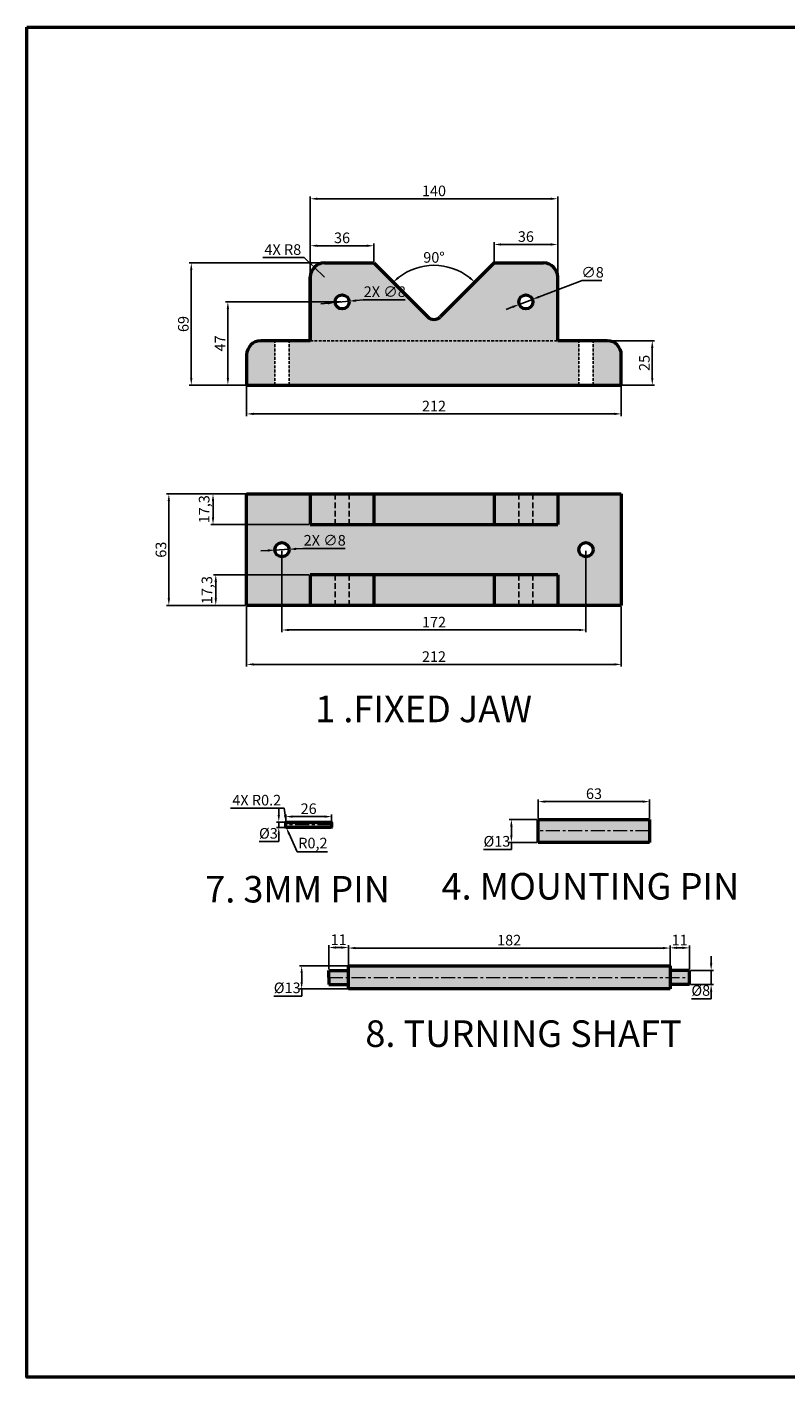
# Model space of a CAD drawing. Units: millimetres. Extents: x -14 to 1073, y -445 to 318.
# Tile 1 of 6: x -14 to 415, y -445 to 318. Entities that reach past the tile are written whole.
import ezdxf

# ---------------------------------------------------------------- set-up
doc = ezdxf.new("R2010")
doc.units = ezdxf.units.MM
doc.header["$LTSCALE"] = 0.5
doc.linetypes.add('CENTER', pattern=[50.8, 31.75, -6.35, 6.35, -6.35])
doc.linetypes.add('HIDDEN', pattern=[9.525, 6.35, -3.175])
for name, color, linetype, lineweight in [('M-CNTR', 1, 'CENTER', 18), ('M-DIMS', 2, 'Continuous', 25), ('M-HATC', 8, 'Continuous', 18), ('M-HIDN', 4, 'HIDDEN', 25), ('M-OUTL', 7, 'Continuous', 50), ('M-TEXT', 3, 'Continuous', 25)]:
    doc.layers.add(name, color=color, linetype=linetype, lineweight=lineweight)
doc.styles.get("Standard").update_dxf_attribs({"font": 'arial.ttf'})
doc.dimstyles.new('ISO-25', dxfattribs={"dimtxt": 6, "dimasz": 4, "dimexe": 1.25, "dimexo": 0.625, "dimtad": 1, "dimtoh": 1, "dimtxsty": 'Standard', "dimcen": 2.5, "dimadec": 0, "dimazin": 0, "dimtfac": 1, "dimtmove": 0, "dimatfit": 3, "dimfxl": 1, "dimarcsym": 0})

# ---------------------------------------------------------------- blocks, each defined once
blk = doc.blocks.new('*D1')
at = {"layer": 'Defpoints', "color": 0, "transparency": 16777216}
for p in [(286.52, 220.97), (146.52, 166.84), (286.52, 166.84)]:
    blk.add_point(p, dxfattribs=at)
at = {"layer": 'M-DIMS', "color": 0, "lineweight": -2, "transparency": 16777216}
for p, q in [((146.52, 167.46), (146.52, 222.22)), ((286.52, 167.46), (286.52, 222.22)), ((150.52, 220.97), (282.52, 220.97))]:
    blk.add_line(p, q, dxfattribs=at)
at = {"layer": 'M-DIMS', "color": 0, "transparency": 16777216}
for points in [[(150.52, 221.64), (150.52, 220.3), (146.52, 220.97)], [(282.52, 221.64), (282.52, 220.3), (286.52, 220.97)]]:
    blk.add_solid(points, dxfattribs=at)
at = {"layer": 'M-DIMS', "color": 0, "transparency": 16777216, "insert": (216.52, 224.66), "char_height": 6, "attachment_point": 5}
blk.add_mtext('140', dxfattribs=at)
blk = doc.blocks.new('*D2')
at = {"layer": 'Defpoints', "color": 0, "transparency": 16777216}
for p in [(146.52, 194.84), (182.52, 194.42), (182.52, 184.67)]:
    blk.add_point(p, dxfattribs=at)
at = {"layer": 'M-DIMS', "color": 0, "lineweight": -2, "transparency": 16777216}
for p, q in [((146.52, 194.22), (146.52, 193.17)), ((150.52, 194.42), (178.52, 194.42)), ((182.52, 185.29), (182.52, 195.67))]:
    blk.add_line(p, q, dxfattribs=at)
at = {"layer": 'M-DIMS', "color": 0, "transparency": 16777216}
for points in [[(150.52, 195.09), (150.52, 193.76), (146.52, 194.42)], [(178.52, 195.09), (178.52, 193.76), (182.52, 194.42)]]:
    blk.add_solid(points, dxfattribs=at)
at = {"layer": 'M-DIMS', "color": 0, "transparency": 16777216, "insert": (164.52, 198.11), "char_height": 6, "attachment_point": 5}
blk.add_mtext('36', dxfattribs=at)
blk = doc.blocks.new('*D3')
at = {"layer": 'Defpoints', "color": 0, "transparency": 16777216}
for p in [(286.52, 195.13), (250.52, 184.67), (286.52, 184.67)]:
    blk.add_point(p, dxfattribs=at)
at = {"layer": 'M-DIMS', "color": 0, "lineweight": -2, "transparency": 16777216}
for p, q in [((250.52, 185.29), (250.52, 196.38)), ((254.52, 195.13), (282.52, 195.13)), ((286.52, 185.29), (286.52, 196.38))]:
    blk.add_line(p, q, dxfattribs=at)
at = {"layer": 'M-DIMS', "color": 0, "transparency": 16777216}
for points in [[(254.52, 195.8), (254.52, 194.47), (250.52, 195.13)], [(282.52, 195.8), (282.52, 194.47), (286.52, 195.13)]]:
    blk.add_solid(points, dxfattribs=at)
at = {"layer": 'M-DIMS', "color": 0, "transparency": 16777216, "insert": (268.52, 198.82), "char_height": 6, "attachment_point": 5}
blk.add_mtext('36', dxfattribs=at)
blk = doc.blocks.new('*D4')
at = {"layer": 'Defpoints', "color": 0, "transparency": 16777216}
for p in [(110.52, 115.67), (322.52, 115.67), (322.52, 99.35)]:
    blk.add_point(p, dxfattribs=at)
at = {"layer": 'M-DIMS', "color": 0, "lineweight": -2, "transparency": 16777216}
for p, q in [((110.52, 115.04), (110.52, 98.1)), ((322.52, 115.04), (322.52, 98.1)), ((114.52, 99.35), (318.52, 99.35))]:
    blk.add_line(p, q, dxfattribs=at)
at = {"layer": 'M-DIMS', "color": 0, "transparency": 16777216}
for points in [[(114.52, 100.02), (114.52, 98.68), (110.52, 99.35)], [(318.52, 100.02), (318.52, 98.68), (322.52, 99.35)]]:
    blk.add_solid(points, dxfattribs=at)
at = {"layer": 'M-DIMS', "color": 0, "transparency": 16777216, "insert": (216.52, 102.99), "char_height": 6, "attachment_point": 5}
blk.add_mtext('212', dxfattribs=at)
blk = doc.blocks.new('*D5')
at = {"layer": 'Defpoints', "color": 0, "transparency": 16777216}
for p in [(307.53, 140.67), (307.53, 115.67), (340.04, 115.67)]:
    blk.add_point(p, dxfattribs=at)
at = {"layer": 'M-DIMS', "color": 0, "lineweight": -2, "transparency": 16777216}
for p, q in [((308.16, 140.67), (341.29, 140.67)), ((340.04, 136.67), (340.04, 119.67)), ((308.16, 115.67), (341.29, 115.67))]:
    blk.add_line(p, q, dxfattribs=at)
at = {"layer": 'M-DIMS', "color": 0, "transparency": 16777216}
for points in [[(339.37, 136.67), (340.7, 136.67), (340.04, 140.67)], [(339.37, 119.67), (340.7, 119.67), (340.04, 115.67)]]:
    blk.add_solid(points, dxfattribs=at)
at = {"layer": 'M-DIMS', "color": 0, "transparency": 16777216, "insert": (336.35, 128.17), "char_height": 6, "attachment_point": 5, "rotation": 90}
blk.add_mtext('25', dxfattribs=at)
blk = doc.blocks.new('*D6')
at = {"layer": 'Defpoints', "color": 0, "transparency": 16777216}
for p in [(164.52, 162.67), (99.9, 115.67), (164.52, 115.67)]:
    blk.add_point(p, dxfattribs=at)
at = {"layer": 'M-DIMS', "color": 0, "lineweight": -2, "transparency": 16777216}
for p, q in [((163.9, 162.67), (98.65, 162.67)), ((99.9, 158.67), (99.9, 119.67)), ((163.9, 115.67), (98.65, 115.67))]:
    blk.add_line(p, q, dxfattribs=at)
at = {"layer": 'M-DIMS', "color": 0, "transparency": 16777216}
for points in [[(99.24, 158.67), (100.57, 158.67), (99.9, 162.67)], [(99.24, 119.67), (100.57, 119.67), (99.9, 115.67)]]:
    blk.add_solid(points, dxfattribs=at)
at = {"layer": 'M-DIMS', "color": 0, "transparency": 16777216, "insert": (96.28, 139.17), "char_height": 6, "attachment_point": 5, "rotation": 90}
blk.add_mtext('47', dxfattribs=at)
blk = doc.blocks.new('*D7')
at = {"layer": 'Defpoints', "color": 0, "transparency": 16777216}
for p in [(168.52, 184.67), (79.19, 115.67), (168.52, 115.67)]:
    blk.add_point(p, dxfattribs=at)
at = {"layer": 'M-DIMS', "color": 0, "lineweight": -2, "transparency": 16777216}
for p, q in [((167.9, 184.67), (77.94, 184.67)), ((79.19, 180.67), (79.19, 119.67)), ((167.9, 115.67), (77.94, 115.67))]:
    blk.add_line(p, q, dxfattribs=at)
at = {"layer": 'M-DIMS', "color": 0, "transparency": 16777216}
for points in [[(78.52, 180.67), (79.85, 180.67), (79.19, 184.67)], [(78.52, 119.67), (79.85, 119.67), (79.19, 115.67)]]:
    blk.add_solid(points, dxfattribs=at)
at = {"layer": 'M-DIMS', "color": 0, "transparency": 16777216, "insert": (75.5, 150.17), "char_height": 6, "attachment_point": 5, "rotation": 90}
blk.add_mtext('69', dxfattribs=at)
blk = doc.blocks.new('*D8')
at = {"layer": 'Defpoints', "color": 0, "transparency": 16777216}
for p in [(182.52, 184.67), (250.52, 184.67), (224.98, 182.24), (212.99, 154.2), (220.06, 154.2)]:
    blk.add_point(p, dxfattribs=at)
at = {"layer": 'M-DIMS', "color": 0, "lineweight": -2, "transparency": 16777216}
blk.add_arc((216.52, 150.67), 32.69, 52.01622, 127.98378, dxfattribs=at)
at = {"layer": 'M-DIMS', "color": 0, "transparency": 16777216}
for points in [[(196.85, 175.93), (195.96, 176.93), (193.41, 173.78)], [(237.08, 176.93), (236.2, 175.93), (239.63, 173.78)]]:
    blk.add_solid(points, dxfattribs=at)
at = {"layer": 'M-DIMS', "color": 0, "transparency": 16777216, "insert": (216.52, 187.04), "char_height": 6, "attachment_point": 5}
blk.add_mtext('90°', dxfattribs=at)
blk = doc.blocks.new('*D9')
at = {"layer": 'Defpoints', "color": 0, "transparency": 16777216}
for p in [(264.78, 161.25), (272.26, 164.09)]:
    blk.add_point(p, dxfattribs=at)
at = {"layer": 'M-DIMS', "color": 0, "lineweight": -2, "transparency": 16777216}
for p, q in [((300.4, 174.76), (276, 165.5)), ((311.5, 174.76), (300.4, 174.76)), ((264.78, 161.25), (272.26, 164.09)), ((261.04, 159.83), (257.3, 158.41))]:
    blk.add_line(p, q, dxfattribs=at)
at = {"layer": 'M-DIMS', "color": 0, "transparency": 16777216}
for points in [[(260.81, 160.45), (261.28, 159.21), (264.78, 161.25)], [(275.77, 166.13), (276.24, 164.88), (272.26, 164.09)]]:
    blk.add_solid(points, dxfattribs=at)
at = {"layer": 'M-DIMS', "color": 0, "transparency": 16777216, "insert": (306.26, 178.61), "char_height": 6, "attachment_point": 5}
blk.add_mtext('∅8', dxfattribs=at)
blk = doc.blocks.new('*D10')
at = {"layer": 'Defpoints', "color": 0, "ltscale": 0.5, "transparency": 16777216}
for p in [(110.52, -8.93), (322.52, -8.93), (322.52, -42.29)]:
    blk.add_point(p, dxfattribs=at)
at = {"layer": 'M-DIMS', "color": 0, "lineweight": -2, "ltscale": 0.5, "transparency": 16777216}
for p, q in [((110.52, -9.55), (110.52, -43.54)), ((322.52, -9.55), (322.52, -43.54)), ((114.52, -42.29), (318.52, -42.29))]:
    blk.add_line(p, q, dxfattribs=at)
at = {"layer": 'M-DIMS', "color": 0, "ltscale": 0.5, "transparency": 16777216}
for points in [[(114.52, -41.63), (114.52, -42.96), (110.52, -42.29)], [(318.52, -41.63), (318.52, -42.96), (322.52, -42.29)]]:
    blk.add_solid(points, dxfattribs=at)
at = {"layer": 'M-DIMS', "color": 0, "ltscale": 0.5, "transparency": 16777216, "insert": (216.52, -38.66), "char_height": 6, "attachment_point": 5}
blk.add_mtext('212', dxfattribs=at)
blk = doc.blocks.new('*D11')
at = {"layer": 'Defpoints', "color": 0, "ltscale": 0.5, "transparency": 16777216}
for p in [(130.52, 22.57), (302.52, 22.57), (302.52, -22.83)]:
    blk.add_point(p, dxfattribs=at)
at = {"layer": 'M-DIMS', "color": 0, "lineweight": -2, "ltscale": 0.5, "transparency": 16777216}
for p, q in [((130.52, 21.95), (130.52, -24.08)), ((302.52, 21.95), (302.52, -24.08)), ((134.52, -22.83), (298.52, -22.83))]:
    blk.add_line(p, q, dxfattribs=at)
at = {"layer": 'M-DIMS', "color": 0, "ltscale": 0.5, "transparency": 16777216}
for points in [[(134.52, -22.16), (134.52, -23.49), (130.52, -22.83)], [(298.52, -22.16), (298.52, -23.49), (302.52, -22.83)]]:
    blk.add_solid(points, dxfattribs=at)
at = {"layer": 'M-DIMS', "color": 0, "ltscale": 0.5, "transparency": 16777216, "insert": (216.52, -19.19), "char_height": 6, "attachment_point": 5}
blk.add_mtext('172', dxfattribs=at)
blk = doc.blocks.new('*D12')
at = {"layer": 'Defpoints', "color": 0, "ltscale": 0.5, "transparency": 16777216}
for p in [(110.52, 54.07), (66.5, -8.93), (110.52, -8.93)]:
    blk.add_point(p, dxfattribs=at)
at = {"layer": 'M-DIMS', "color": 0, "lineweight": -2, "ltscale": 0.5, "transparency": 16777216}
for p, q in [((109.9, 54.07), (65.25, 54.07)), ((66.5, 50.07), (66.5, -4.93)), ((109.9, -8.93), (65.25, -8.93))]:
    blk.add_line(p, q, dxfattribs=at)
at = {"layer": 'M-DIMS', "color": 0, "ltscale": 0.5, "transparency": 16777216}
for points in [[(65.84, 50.07), (67.17, 50.07), (66.5, 54.07)], [(65.84, -4.93), (67.17, -4.93), (66.5, -8.93)]]:
    blk.add_solid(points, dxfattribs=at)
at = {"layer": 'M-DIMS', "color": 0, "ltscale": 0.5, "transparency": 16777216, "insert": (62.81, 22.57), "char_height": 6, "attachment_point": 5, "rotation": 90}
blk.add_mtext('63', dxfattribs=at)
blk = doc.blocks.new('*D13')
at = {"layer": 'Defpoints', "color": 0, "ltscale": 0.5, "transparency": 16777216}
for p in [(146.52, 54.07), (91.5, 36.77), (146.52, 36.77)]:
    blk.add_point(p, dxfattribs=at)
at = {"layer": 'M-DIMS', "color": 0, "lineweight": -2, "ltscale": 0.5, "transparency": 16777216}
for p, q in [((145.9, 54.07), (90.25, 54.07)), ((91.5, 50.07), (91.5, 40.77)), ((145.9, 36.77), (90.25, 36.77))]:
    blk.add_line(p, q, dxfattribs=at)
at = {"layer": 'M-DIMS', "color": 0, "ltscale": 0.5, "transparency": 16777216}
for points in [[(90.83, 50.07), (92.16, 50.07), (91.5, 54.07)], [(90.83, 40.77), (92.16, 40.77), (91.5, 36.77)]]:
    blk.add_solid(points, dxfattribs=at)
at = {"layer": 'M-DIMS', "color": 0, "ltscale": 0.5, "transparency": 16777216, "insert": (87.27, 45.42), "char_height": 6, "attachment_point": 5, "rotation": 90}
blk.add_mtext('17,3', dxfattribs=at)
blk = doc.blocks.new('*D14')
at = {"layer": 'Defpoints', "color": 0, "ltscale": 0.5, "transparency": 16777216}
for p in [(146.52, 8.37), (93.06, -8.93), (110.52, -8.93)]:
    blk.add_point(p, dxfattribs=at)
at = {"layer": 'M-DIMS', "color": 0, "lineweight": -2, "ltscale": 0.5, "transparency": 16777216}
for p, q in [((145.9, 8.37), (91.81, 8.37)), ((93.06, 4.37), (93.06, -4.93)), ((109.9, -8.93), (91.81, -8.93))]:
    blk.add_line(p, q, dxfattribs=at)
at = {"layer": 'M-DIMS', "color": 0, "ltscale": 0.5, "transparency": 16777216}
for points in [[(92.39, 4.37), (93.73, 4.37), (93.06, 8.37)], [(92.39, -4.93), (93.73, -4.93), (93.06, -8.93)]]:
    blk.add_solid(points, dxfattribs=at)
at = {"layer": 'M-DIMS', "color": 0, "ltscale": 0.5, "transparency": 16777216, "insert": (88.83, -0.28), "char_height": 6, "attachment_point": 5, "rotation": 90}
blk.add_mtext('17,3', dxfattribs=at)
blk = doc.blocks.new('*D28')
at = {"layer": 'Defpoints', "color": 0, "ltscale": 0.5, "transparency": 16777216}
for p in [(158.61, -128.34), (132.61, -132.94), (158.61, -132.94)]:
    blk.add_point(p, dxfattribs=at)
at = {"layer": 'M-DIMS', "color": 0, "lineweight": -2, "ltscale": 0.5, "transparency": 16777216}
for p, q in [((132.61, -132.31), (132.61, -127.09)), ((136.61, -128.34), (154.61, -128.34)), ((158.61, -132.31), (158.61, -127.09))]:
    blk.add_line(p, q, dxfattribs=at)
at = {"layer": 'M-DIMS', "color": 0, "ltscale": 0.5, "transparency": 16777216}
for points in [[(136.61, -127.68), (136.61, -129.01), (132.61, -128.34)], [(154.61, -127.68), (154.61, -129.01), (158.61, -128.34)]]:
    blk.add_solid(points, dxfattribs=at)
at = {"layer": 'M-DIMS', "color": 0, "ltscale": 0.5, "transparency": 16777216, "insert": (145.61, -124.65), "char_height": 6, "attachment_point": 5}
blk.add_mtext('26', dxfattribs=at)
blk = doc.blocks.new('*D29')
at = {"layer": 'Defpoints', "color": 0, "ltscale": 0.5, "transparency": 16777216}
for p in [(128.7, -134.44), (133.54, -131.44), (133.54, -134.44)]:
    blk.add_point(p, dxfattribs=at)
at = {"layer": 'M-DIMS', "color": 0, "lineweight": -2, "ltscale": 0.5, "transparency": 16777216}
for p, q in [((128.7, -127.44), (128.7, -123.44)), ((132.91, -131.44), (127.45, -131.44)), ((132.91, -134.44), (127.45, -134.44)), ((128.7, -131.44), (128.7, -134.44)), ((128.7, -142.44), (117.61, -142.44)), ((128.7, -138.44), (128.7, -142.44))]:
    blk.add_line(p, q, dxfattribs=at)
at = {"layer": 'M-DIMS', "color": 0, "ltscale": 0.5, "transparency": 16777216}
for points in [[(128.03, -127.44), (129.36, -127.44), (128.7, -131.44)], [(128.03, -138.44), (129.36, -138.44), (128.7, -134.44)]]:
    blk.add_solid(points, dxfattribs=at)
at = {"layer": 'M-DIMS', "color": 0, "ltscale": 0.5, "transparency": 16777216, "insert": (122.84, -138.58), "char_height": 6, "attachment_point": 5}
blk.add_mtext('%%C3', dxfattribs=at)
blk = doc.blocks.new('*D30')
at = {"layer": 'Defpoints', "color": 0, "ltscale": 0.5, "transparency": 16777216}
for p in [(132.81, -134.24), (132.89, -134.42)]:
    blk.add_point(p, dxfattribs=at)
at = {"layer": 'M-DIMS', "color": 0, "lineweight": -2, "ltscale": 0.5, "transparency": 16777216}
for p, q in [((132.81, -134.24), (132.89, -134.42)), ((139.09, -148.31), (134.52, -138.07)), ((156.32, -148.31), (139.09, -148.31))]:
    blk.add_line(p, q, dxfattribs=at)
blk.add_arc((132.81, -134.24), 0.2, 270, 294.08317, dxfattribs=at)
at = {"layer": 'M-DIMS', "color": 0, "ltscale": 0.5, "transparency": 16777216}
blk.add_solid([(135.13, -137.8), (133.91, -138.35), (132.89, -134.42)], dxfattribs=at)
at = {"layer": 'M-DIMS', "color": 0, "ltscale": 0.5, "transparency": 16777216, "insert": (148.02, -144.08), "char_height": 6, "attachment_point": 5}
blk.add_mtext('R0,2', dxfattribs=at)
blk = doc.blocks.new('*D31')
at = {"layer": 'Defpoints', "color": 0, "ltscale": 0.5, "transparency": 16777216}
for p in [(338.56, -119.86), (275.56, -129.94), (338.56, -129.94)]:
    blk.add_point(p, dxfattribs=at)
at = {"layer": 'M-DIMS', "color": 0, "lineweight": -2, "ltscale": 0.5, "transparency": 16777216}
for p, q in [((275.56, -129.32), (275.56, -118.61)), ((279.56, -119.86), (334.56, -119.86)), ((338.56, -129.32), (338.56, -118.61))]:
    blk.add_line(p, q, dxfattribs=at)
at = {"layer": 'M-DIMS', "color": 0, "ltscale": 0.5, "transparency": 16777216}
for points in [[(279.56, -119.2), (279.56, -120.53), (275.56, -119.86)], [(334.56, -119.2), (334.56, -120.53), (338.56, -119.86)]]:
    blk.add_solid(points, dxfattribs=at)
at = {"layer": 'M-DIMS', "color": 0, "ltscale": 0.5, "transparency": 16777216, "insert": (307.06, -116.17), "char_height": 6, "attachment_point": 5}
blk.add_mtext('63', dxfattribs=at)
blk = doc.blocks.new('*D32')
at = {"layer": 'Defpoints', "color": 0, "ltscale": 0.5, "transparency": 16777216}
for p in [(275.56, -129.94), (260.32, -142.94), (275.56, -142.94)]:
    blk.add_point(p, dxfattribs=at)
at = {"layer": 'M-DIMS', "color": 0, "lineweight": -2, "ltscale": 0.5, "transparency": 16777216}
for p, q in [((274.94, -129.94), (259.07, -129.94)), ((260.32, -133.94), (260.32, -138.94)), ((274.94, -142.94), (259.07, -142.94)), ((260.32, -142.94), (260.32, -146.94)), ((260.32, -146.94), (244.57, -146.94))]:
    blk.add_line(p, q, dxfattribs=at)
at = {"layer": 'M-DIMS', "color": 0, "ltscale": 0.5, "transparency": 16777216}
for points in [[(259.65, -133.94), (260.99, -133.94), (260.32, -129.94)], [(259.65, -138.94), (260.99, -138.94), (260.32, -142.94)]]:
    blk.add_solid(points, dxfattribs=at)
at = {"layer": 'M-DIMS', "color": 0, "ltscale": 0.5, "transparency": 16777216, "insert": (252.13, -143.08), "char_height": 6, "attachment_point": 5}
blk.add_mtext('%%C13', dxfattribs=at)
blk = doc.blocks.new('*D33')
at = {"layer": 'Defpoints', "color": 0, "ltscale": 0.5, "transparency": 16777216}
for p in [(168.07, -202.36), (157.07, -215.28), (168.07, -215.28)]:
    blk.add_point(p, dxfattribs=at)
at = {"layer": 'M-DIMS', "color": 0, "lineweight": -2, "ltscale": 0.5, "transparency": 16777216}
for p, q in [((157.07, -214.66), (157.07, -201.11)), ((161.07, -202.36), (164.07, -202.36)), ((168.07, -214.66), (168.07, -201.11))]:
    blk.add_line(p, q, dxfattribs=at)
at = {"layer": 'M-DIMS', "color": 0, "ltscale": 0.5, "transparency": 16777216}
for points in [[(161.07, -201.7), (161.07, -203.03), (157.07, -202.36)], [(164.07, -201.7), (164.07, -203.03), (168.07, -202.36)]]:
    blk.add_solid(points, dxfattribs=at)
at = {"layer": 'M-DIMS', "color": 0, "ltscale": 0.5, "transparency": 16777216, "insert": (162.57, -198.73), "char_height": 6, "attachment_point": 5}
blk.add_mtext('11', dxfattribs=at)
blk = doc.blocks.new('*D34')
at = {"layer": 'Defpoints', "color": 0, "ltscale": 0.5, "transparency": 16777216}
for p in [(350.07, -202.66), (168.07, -207.89), (350.07, -212.78)]:
    blk.add_point(p, dxfattribs=at)
at = {"layer": 'M-DIMS', "color": 0, "lineweight": -2, "ltscale": 0.5, "transparency": 16777216}
for p, q in [((168.07, -207.26), (168.07, -201.41)), ((172.07, -202.66), (346.07, -202.66)), ((350.07, -212.16), (350.07, -201.41))]:
    blk.add_line(p, q, dxfattribs=at)
at = {"layer": 'M-DIMS', "color": 0, "ltscale": 0.5, "transparency": 16777216}
for points in [[(172.07, -201.99), (172.07, -203.33), (168.07, -202.66)], [(346.07, -201.99), (346.07, -203.33), (350.07, -202.66)]]:
    blk.add_solid(points, dxfattribs=at)
at = {"layer": 'M-DIMS', "color": 0, "ltscale": 0.5, "transparency": 16777216, "insert": (259.07, -198.97), "char_height": 6, "attachment_point": 5}
blk.add_mtext('182', dxfattribs=at)
blk = doc.blocks.new('*D35')
at = {"layer": 'Defpoints', "color": 0, "ltscale": 0.5, "transparency": 16777216}
for p in [(361.07, -202.54), (350.07, -215.28), (361.07, -215.28)]:
    blk.add_point(p, dxfattribs=at)
at = {"layer": 'M-DIMS', "color": 0, "lineweight": -2, "ltscale": 0.5, "transparency": 16777216}
for p, q in [((350.07, -214.66), (350.07, -201.29)), ((354.07, -202.54), (357.07, -202.54)), ((361.07, -214.66), (361.07, -201.29))]:
    blk.add_line(p, q, dxfattribs=at)
at = {"layer": 'M-DIMS', "color": 0, "ltscale": 0.5, "transparency": 16777216}
for points in [[(354.07, -201.88), (354.07, -203.21), (350.07, -202.54)], [(357.07, -201.88), (357.07, -203.21), (361.07, -202.54)]]:
    blk.add_solid(points, dxfattribs=at)
at = {"layer": 'M-DIMS', "color": 0, "ltscale": 0.5, "transparency": 16777216, "insert": (355.57, -198.9), "char_height": 6, "attachment_point": 5}
blk.add_mtext('11', dxfattribs=at)
blk = doc.blocks.new('*D36')
at = {"layer": 'Defpoints', "color": 0, "ltscale": 0.5, "transparency": 16777216}
for p in [(361.07, -215.28), (361.07, -223.28), (373.35, -223.28)]:
    blk.add_point(p, dxfattribs=at)
at = {"layer": 'M-DIMS', "color": 0, "lineweight": -2, "ltscale": 0.5, "transparency": 16777216}
for p, q in [((373.35, -211.28), (373.35, -207.28)), ((361.7, -215.28), (374.6, -215.28)), ((373.35, -215.28), (373.35, -223.28)), ((361.7, -223.28), (374.6, -223.28)), ((373.35, -227.28), (373.35, -231.28)), ((373.35, -231.28), (362.25, -231.28))]:
    blk.add_line(p, q, dxfattribs=at)
at = {"layer": 'M-DIMS', "color": 0, "ltscale": 0.5, "transparency": 16777216}
for points in [[(372.68, -211.28), (374.01, -211.28), (373.35, -215.28)], [(372.68, -227.28), (374.01, -227.28), (373.35, -223.28)]]:
    blk.add_solid(points, dxfattribs=at)
at = {"layer": 'M-DIMS', "color": 0, "ltscale": 0.5, "transparency": 16777216, "insert": (367.48, -227.43), "char_height": 6, "attachment_point": 5}
blk.add_mtext('%%C8', dxfattribs=at)
blk = doc.blocks.new('*D37')
at = {"layer": 'Defpoints', "color": 0, "ltscale": 0.5, "transparency": 16777216}
for p in [(202.48, -212.78), (141.66, -225.78), (202.48, -225.78)]:
    blk.add_point(p, dxfattribs=at)
at = {"layer": 'M-DIMS', "color": 0, "lineweight": -2, "ltscale": 0.5, "transparency": 16777216}
for p, q in [((201.85, -212.78), (140.41, -212.78)), ((141.66, -216.78), (141.66, -221.78)), ((201.85, -225.78), (140.41, -225.78)), ((141.66, -225.78), (141.66, -229.78)), ((141.66, -229.78), (125.91, -229.78))]:
    blk.add_line(p, q, dxfattribs=at)
at = {"layer": 'M-DIMS', "color": 0, "ltscale": 0.5, "transparency": 16777216}
for points in [[(140.99, -216.78), (142.33, -216.78), (141.66, -212.78)], [(140.99, -221.78), (142.33, -221.78), (141.66, -225.78)]]:
    blk.add_solid(points, dxfattribs=at)
at = {"layer": 'M-DIMS', "color": 0, "ltscale": 0.5, "transparency": 16777216, "insert": (133.47, -225.93), "char_height": 6, "attachment_point": 5}
blk.add_mtext('%%C13', dxfattribs=at)
blk = doc.blocks.new('*D81')
at = {"layer": 'Defpoints', "color": 0, "ltscale": 0.5, "transparency": 16777216}
for p in [(148.78, 182.24), (154.52, 176.67)]:
    blk.add_point(p, dxfattribs=at)
at = {"layer": 'M-DIMS', "color": 0, "lineweight": -2, "ltscale": 0.5, "transparency": 16777216}
for p, q in [((119.59, 187.81), (143.04, 187.81)), ((143.04, 187.81), (145.91, 185.02)), ((154.52, 176.67), (148.78, 182.24))]:
    blk.add_line(p, q, dxfattribs=at)
at = {"layer": 'M-DIMS', "color": 0, "ltscale": 0.5, "transparency": 16777216}
blk.add_solid([(146.37, 185.5), (145.44, 184.54), (148.78, 182.24)], dxfattribs=at)
at = {"layer": 'M-DIMS', "color": 0, "ltscale": 0.5, "transparency": 16777216, "insert": (131, 191.49), "char_height": 6, "attachment_point": 5}
blk.add_mtext('4X R8', dxfattribs=at)
blk = doc.blocks.new('*D82')
at = {"layer": 'Defpoints', "color": 0, "ltscale": 0.5, "transparency": 16777216}
for p in [(160.54, 162.29), (168.5, 163.05)]:
    blk.add_point(p, dxfattribs=at)
at = {"layer": 'M-DIMS', "color": 0, "lineweight": -2, "ltscale": 0.5, "transparency": 16777216}
for p, q in [((156.56, 161.9), (152.58, 161.52)), ((160.54, 162.29), (168.5, 163.05)), ((176.47, 163.81), (172.49, 163.43)), ((200.24, 163.81), (176.47, 163.81))]:
    blk.add_line(p, q, dxfattribs=at)
at = {"layer": 'M-DIMS', "color": 0, "ltscale": 0.5, "transparency": 16777216}
for points in [[(156.49, 162.57), (156.62, 161.24), (160.54, 162.29)], [(172.42, 164.09), (172.55, 162.77), (168.5, 163.05)]]:
    blk.add_solid(points, dxfattribs=at)
at = {"layer": 'M-DIMS', "color": 0, "ltscale": 0.5, "transparency": 16777216, "insert": (188.67, 167.67), "char_height": 6, "attachment_point": 5}
blk.add_mtext('2X ∅8', dxfattribs=at)
blk = doc.blocks.new('*D83')
at = {"layer": 'Defpoints', "color": 0, "ltscale": 0.5, "transparency": 16777216}
for p in [(126.53, 22.35), (134.52, 22.8)]:
    blk.add_point(p, dxfattribs=at)
at = {"layer": 'M-DIMS', "color": 0, "lineweight": -2, "ltscale": 0.5, "transparency": 16777216}
for p, q in [((142.5, 23.26), (138.51, 23.03)), ((166.28, 23.26), (142.5, 23.26)), ((122.53, 22.12), (118.54, 21.89)), ((126.53, 22.35), (134.52, 22.8))]:
    blk.add_line(p, q, dxfattribs=at)
at = {"layer": 'M-DIMS', "color": 0, "ltscale": 0.5, "transparency": 16777216}
for points in [[(138.47, 23.69), (138.55, 22.36), (134.52, 22.8)], [(122.5, 22.78), (122.57, 21.45), (126.53, 22.35)]]:
    blk.add_solid(points, dxfattribs=at)
at = {"layer": 'M-DIMS', "color": 0, "ltscale": 0.5, "transparency": 16777216, "insert": (154.7, 27.11), "char_height": 6, "attachment_point": 5}
blk.add_mtext('2X ∅8', dxfattribs=at)
blk = doc.blocks.new('*D96')
at = {"layer": 'Defpoints', "color": 0, "ltscale": 0.5, "transparency": 16777216}
for p in [(132.78, -131.44), (132.81, -131.64)]:
    blk.add_point(p, dxfattribs=at)
at = {"layer": 'M-DIMS', "color": 0, "lineweight": -2, "ltscale": 0.5, "transparency": 16777216}
for p, q in [((101.36, -123.51), (131.72, -123.51)), ((131.72, -123.51), (132.25, -127.48)), ((132.81, -131.64), (132.78, -131.44))]:
    blk.add_line(p, q, dxfattribs=at)
at = {"layer": 'M-DIMS', "color": 0, "ltscale": 0.5, "transparency": 16777216}
blk.add_solid([(132.91, -127.39), (131.59, -127.56), (132.78, -131.44)], dxfattribs=at)
at = {"layer": 'M-DIMS', "color": 0, "ltscale": 0.5, "transparency": 16777216, "insert": (116.23, -119.82), "char_height": 6, "attachment_point": 5}
blk.add_mtext('4X R0.2', dxfattribs=at)

msp = doc.modelspace()

# ---------------------------------------------------------------- hatches: boundary and pattern name
at = {"layer": 'M-HATC', "ltscale": 0.5}
h = msp.add_hatch(color=256, dxfattribs=at)
h.set_gradient(color1=(41, 49, 137), color2=(41, 49, 137), tint=1)
h.paths.add_polyline_path([(182.5216, 184.6668), (154.5216, 184.6668, 0.41421356), (146.5216, 176.6668), (146.5216, 140.6668), (286.5216, 140.6668), (286.5216, 176.6668, 0.41421356), (278.5216, 184.6668), (250.5216, 184.6668), (220.0571, 154.2024, -0.41421356), (212.9861, 154.2024)])
h.paths.add_polyline_path([(160.5216, 162.6668, -1), (168.5216, 162.6668, -1)], flags=16)
h.paths.add_polyline_path([(272.5216, 162.6668, -1), (264.5216, 162.6668, -1)], flags=16)
h.paths.add_polyline_path([(298.5216, 140.6668), (286.5216, 140.6668), (146.5216, 140.6668), (134.5216, 140.6668), (134.5216, 115.6668), (298.5216, 115.6668)])
h.paths.add_polyline_path([(126.5216, 140.6668), (118.5216, 140.6668, 0.41421356), (110.5216, 132.6668), (110.5216, 115.6668), (126.5216, 115.6668)])
h.paths.add_polyline_path([(322.5216, 132.6668, 0.41421356), (314.5216, 140.6668), (306.5216, 140.6668), (306.5216, 115.6668), (322.5216, 115.6668)])
h = msp.add_hatch(color=256, dxfattribs=at)
h.set_gradient(color1=(69, 84, 165), color2=(69, 84, 165), tint=1)
h.paths.add_polyline_path([(322.5216, 54.0737), (286.5216, 54.0737), (286.5216, 36.7737), (146.5216, 36.7737), (146.5216, 54.0737), (110.5216, 54.0737), (110.5216, -8.9263), (146.5216, -8.9263), (146.5216, 8.3737), (286.5216, 8.3737), (286.5216, -8.9263), (322.5216, -8.9263)])
h.paths.add_polyline_path([(306.5216, 22.5737, -1), (298.5216, 22.5737, -1)], flags=16)
h.paths.add_polyline_path([(126.5216, 22.5737, -1), (134.5216, 22.5737, -1)], flags=16)
h.paths.add_polyline_path([(250.5216, 54.0737), (182.5216, 54.0737), (182.5216, 36.7737), (250.5216, 36.7737)], flags=17)
h.paths.add_polyline_path([(182.5216, 54.0737), (168.5216, 54.0737), (168.5216, 36.7737), (182.5216, 36.7737)], flags=17)
h.paths.add_polyline_path([(168.5216, 54.0737), (160.5216, 54.0737), (160.5216, 36.7737), (168.5216, 36.7737)], flags=17)
h.paths.add_polyline_path([(160.5216, 54.0737), (146.5216, 54.0737), (146.5216, 36.7737), (160.5216, 36.7737)], flags=17)
h.paths.add_polyline_path([(264.5216, 54.0737), (250.5216, 54.0737), (250.5216, 36.7737), (264.5216, 36.7737)], flags=17)
h.paths.add_polyline_path([(272.5216, 54.0737), (264.5216, 54.0737), (264.5216, 36.7737), (272.5216, 36.7737)], flags=17)
h.paths.add_polyline_path([(286.5216, 54.0737), (272.5216, 54.0737), (272.5216, 36.7737), (286.5216, 36.7737)], flags=17)
h.paths.add_polyline_path([(160.5216, 8.3737), (146.5216, 8.3737), (146.5216, -8.9263), (160.5216, -8.9263)], flags=17)
h.paths.add_polyline_path([(168.5216, 8.3737), (160.5216, 8.3737), (160.5216, -8.9263), (168.5216, -8.9263)], flags=17)
h.paths.add_polyline_path([(182.5216, 8.3737), (168.5216, 8.3737), (168.5216, -8.9263), (182.5216, -8.9263)], flags=17)
h.paths.add_polyline_path([(250.5216, 8.3737), (182.5216, 8.3737), (182.5216, -8.9263), (250.5216, -8.9263)], flags=17)
h.paths.add_polyline_path([(264.5216, 8.3737), (250.5216, 8.3737), (250.5216, -8.9263), (264.5216, -8.9263)], flags=17)
h.paths.add_polyline_path([(272.5216, 8.3737), (264.5216, 8.3737), (264.5216, -8.9263), (272.5216, -8.9263)], flags=17)
h.paths.add_polyline_path([(286.5216, 8.3737), (272.5216, 8.3737), (272.5216, -8.9263), (286.5216, -8.9263)], flags=17)
h = msp.add_hatch(color=256, dxfattribs=at)
h.set_gradient(color1=(221, 179, 212), color2=(221, 179, 212), tint=1)
h.paths.add_polyline_path([(158.6052, -132.939), (158.6052, -131.639, 0.41421356), (158.4052, -131.439), (132.8052, -131.439, 0.41421356), (132.6052, -131.639), (132.6052, -132.939)])
h.paths.add_polyline_path([(132.6052, -132.939), (132.6052, -134.239, 0.41421356), (132.8052, -134.439), (158.4052, -134.439, 0.41421356), (158.6052, -134.239), (158.6052, -132.939)])
h = msp.add_hatch(color=256, dxfattribs=at)
h.set_gradient(color1=(128, 128, 128), color2=(128, 128, 128), tint=1)
h.paths.add_polyline_path([(338.5603, -136.4411), (275.5603, -136.4411), (275.5603, -142.9411), (338.5603, -142.9411)])
h.paths.add_polyline_path([(338.5603, -129.9411), (275.5603, -129.9411), (275.5603, -136.4411), (338.5603, -136.4411)])
h = msp.add_hatch(color=256, dxfattribs=at)
h.set_gradient(color1=(128, 128, 128), color2=(192, 192, 192), tint=1, name='INVCYLINDER')
h.paths.add_polyline_path([(350.0728, -212.7819), (168.0728, -212.7819), (168.0728, -219.2819), (350.0728, -219.2819)])
h.paths.add_polyline_path([(350.0728, -219.2819), (168.0728, -219.2819), (168.0728, -225.7819), (350.0728, -225.7819)])
h.paths.add_polyline_path([(168.0728, -215.2819), (157.0728, -215.2819), (157.0728, -219.2819), (168.0728, -219.2819)])
h.paths.add_polyline_path([(168.0728, -219.2819), (157.0728, -219.2819), (157.0728, -223.2819), (168.0728, -223.2819)])
h = msp.add_hatch(color=256, dxfattribs=at)
h.set_gradient(color1=(128, 128, 128), color2=(192, 192, 192), tint=1, name='INVCYLINDER')
h.paths.add_polyline_path([(361.0728, -223.2819), (361.0728, -215.2819), (350.0728, -215.2819), (350.0728, -223.2819)])

# ---------------------------------------------------------------- linework, layer by layer
at = {"layer": 'M-CNTR', "ltscale": 0.5}
for p, q in [((158.6052, -132.939), (132.6052, -132.939)), ((338.5603, -136.4411), (275.5603, -136.4411)), ((157.0728, -219.2819), (350.0728, -219.2819)), ((157.0728, -219.2819), (361.0728, -219.2819))]:
    msp.add_line(p, q, dxfattribs=at)
at = {"layer": 'M-HIDN', "ltscale": 0.5}
for p, q in [((126.5216, 115.6668), (126.5216, 140.6668)), ((134.5216, 115.6668), (134.5216, 140.6668)), ((146.5216, 140.6668), (286.5216, 140.6668)), ((298.5216, 115.6668), (298.5216, 140.6668)), ((306.5216, 115.6668), (306.5216, 140.6668))]:
    msp.add_line(p, q, dxfattribs=at)
at = {"layer": 'M-HIDN'}
for p, q in [((160.5216, 54.0737), (160.5216, 36.7737)), ((168.5216, 54.0737), (168.5216, 36.7737)), ((264.5216, 54.0737), (264.5216, 36.7737)), ((272.5216, 54.0737), (272.5216, 36.7737)), ((160.5216, 8.3737), (160.5216, -8.9263)), ((168.5216, 8.3737), (168.5216, -8.9263)), ((264.5216, 8.3737), (264.5216, -8.9263)), ((272.5216, 8.3737), (272.5216, -8.9263))]:
    msp.add_line(p, q, dxfattribs=at)
at = {"layer": 'M-OUTL'}
for p, q in [((154.5216, 184.6668), (182.5216, 184.6668)), ((182.5216, 184.6668), (212.9861, 154.2024)), ((250.5216, 184.6668), (220.0571, 154.2024)), ((250.5216, 184.6668), (278.5216, 184.6668)), ((146.5216, 140.6668), (146.5216, 176.6668)), ((146.5216, 140.6668), (146.5216, 176.6668)), ((146.5216, 176.6668), (146.5216, 140.6668)), ((286.5216, 140.6668), (286.5216, 176.6668)), ((146.5216, 140.6668), (118.5216, 140.6668)), ((314.5216, 140.6668), (286.5216, 140.6668)), ((110.5216, 132.6668), (110.5216, 115.6668)), ((322.5216, 115.6668), (322.5216, 132.6668)), ((110.5216, 115.6668), (322.5216, 115.6668)), ((110.5216, 54.0737), (322.5216, 54.0737)), ((110.5216, -8.9263), (110.5216, 54.0737)), ((146.5216, 54.0737), (146.5216, 36.7737)), ((182.5216, 54.0737), (182.5216, 36.7737)), ((250.5216, 54.0737), (250.5216, 36.7737)), ((286.5216, 54.0737), (286.5216, 36.7737)), ((322.5216, 54.0737), (322.5216, -8.9263)), ((146.5216, 36.7737), (286.5216, 36.7737)), ((146.5216, 8.3737), (146.5216, -8.9263)), ((286.5216, 8.3737), (146.5216, 8.3737)), ((182.5216, 8.3737), (182.5216, -8.9263)), ((250.5216, 8.3737), (250.5216, -8.9263)), ((286.5216, 8.3737), (286.5216, -8.9263)), ((322.5216, -8.9263), (110.5216, -8.9263))]:
    msp.add_line(p, q, dxfattribs=at)
at = {"layer": 'M-OUTL', "ltscale": 0.5}
for p, q in [((132.6052, -134.239), (132.6052, -131.639)), ((132.8052, -131.439), (158.4052, -131.439)), ((158.4052, -134.439), (132.8052, -134.439)), ((158.6052, -131.639), (158.6052, -134.239)), ((275.5603, -129.9411), (338.5603, -129.9411)), ((275.5603, -142.9411), (275.5603, -129.9411)), ((338.5603, -129.9411), (338.5603, -142.9411)), ((338.5603, -142.9411), (275.5603, -142.9411)), ((168.0728, -212.7819), (350.0728, -212.7819)), ((168.0728, -225.7819), (168.0728, -212.7819)), ((350.0728, -212.7819), (350.0728, -225.7819)), ((157.0728, -219.2819), (157.0728, -215.2819)), ((157.0728, -215.2819), (168.0728, -215.2819)), ((157.0728, -219.2819), (157.0728, -223.2819)), ((168.0728, -223.2819), (168.0728, -215.2819)), ((361.0728, -215.2819), (350.0728, -215.2819)), ((361.0728, -223.2819), (361.0728, -215.2819)), ((157.0728, -223.2819), (168.0728, -223.2819)), ((350.0728, -225.7819), (168.0728, -225.7819)), ((361.0728, -223.2819), (350.0728, -223.2819))]:
    msp.add_line(p, q, dxfattribs=at)
msp.add_lwpolyline([(-13.7695, 318.0907), (1072.7514, 318.0907), (1072.7514, -445.1795), (-13.7695, -445.1795)], close=True, dxfattribs=at)
at = {"layer": 'M-OUTL'}
for centre in [(164.5216, 162.6668), (268.5216, 162.6668), (130.5216, 22.5737), (302.5216, 22.5737)]:
    msp.add_circle(centre, 4, dxfattribs=at)
for centre, radius, start, end in [((154.5216, 176.6668), 8, 90, 180), ((278.5216, 176.6668), 8, 0, 90), ((216.5216, 157.7379), 5, 225, 315), ((118.5216, 132.6668), 8, 90, 180), ((314.5216, 132.6668), 8, 0, 90)]:
    msp.add_arc(centre, radius, start, end, dxfattribs=at)
at = {"layer": 'M-OUTL', "ltscale": 0.5}
for centre, start, end in [((132.8052, -131.639), 90, 180), ((132.8052, -134.239), 180, 270), ((158.4052, -131.639), 0, 90), ((158.4052, -134.239), 270, 0)]:
    msp.add_arc(centre, 0.2, start, end, dxfattribs=at)

# ---------------------------------------------------------------- texts
at = {"layer": 'M-TEXT', "ltscale": 0.5, "char_height": 15, "attachment_point": 1}
for s, width, insert in [('\\pxqc;1 .FIXED JAW', 165.349413, (127.9745, -59.9711)), ('\\pxqc;4. MOUNTING PIN', 179.382141, (215.3142, -160.2513)), ('\\pxqc;7. 3MM PIN', 165.349413, (56.6453, -161.8991)), ('\\pxqc;8. TURNING SHAFT', 198.556311, (167.9041, -243.5504))]:
    msp.add_mtext_dynamic_manual_height_columns(s, width=width, gutter_width=12.5, heights=[0], dxfattribs=dict(at, insert=insert))

# ---------------------------------------------------------------- dimensions: what is measured, and where the dimension line sits
at = {"layer": 'M-DIMS'}
for base, p1, p2, picture, middle in [((286.5216, 220.9685), (146.5216, 166.8383), (286.5216, 166.8383), '*D1', (216.5216, 224.6569)), ((182.5216, 194.4223), (146.5216, 194.8409), (182.5216, 184.6668), '*D2', (164.5216, 198.1128)), ((286.5216, 195.1333), (250.5216, 184.6668), (286.5216, 184.6668), '*D3', (268.5216, 198.8238)), ((322.5216, 99.3508), (110.5216, 115.6668), (322.5216, 115.6668), '*D4', (216.5216, 102.9881))]:
    dim = msp.add_linear_dim(base=base, p1=p1, p2=p2, dimstyle='ISO-25', override={"dimclrd": 0, "dimclre": 0, "dimclrt": 0}, dxfattribs=at)
    dim.commit()
    dim.dimension.update_dxf_attribs({"geometry": picture, "text_midpoint": middle})
at = {"layer": 'M-DIMS', "ltscale": 0.5}
for center, mpoint, override, picture, middle in [((154.5216, 176.6668), (148.7784, 182.236), {"dimdec": 0, "dimlfac": 1, "dimrnd": 0, "dimzin": 0, "dimdsep": 46, "dimlunit": 2}, '*D81', (130.9996, 191.4937)), ((132.8052, -131.639), (132.7787, -131.4408), {"dimdec": 1, "dimlfac": 1, "dimrnd": 0, "dimzin": 0, "dimdsep": 46, "dimlunit": 2}, '*D96', (116.2265, -119.8226))]:
    dim = msp.add_radius_dim(center=center, mpoint=mpoint, text='4X <>', dimstyle='ISO-25', override=override, dxfattribs=at)
    dim.commit()
    dim.dimension.update_dxf_attribs({"geometry": picture, "text_midpoint": middle})
at = {"layer": 'M-DIMS'}
dim = msp.add_angular_dim_2l(base=(224.9812, 182.2383), line1=((250.5216, 184.6668), (220.0571, 154.2024)), line2=((182.5216, 184.6668), (212.9861, 154.2024)), dimstyle='ISO-25', override={"dimclrd": 0, "dimclre": 0, "dimclrt": 0}, dxfattribs=at)
dim.commit()
dim.dimension.update_dxf_attribs({"geometry": '*D8', "text_midpoint": (216.5216, 187.0405)})
for base, p1, p2, picture, middle in [((79.1867, 115.6668), (168.5216, 184.6668), (168.5216, 115.6668), '*D7', (75.4983, 150.1668)), ((99.9036, 115.6668), (164.5216, 162.6668), (164.5216, 115.6668), '*D6', (96.2786, 139.1668)), ((340.0368, 115.6668), (307.534, 140.6668), (307.534, 115.6668), '*D5', (336.3484, 128.1668))]:
    dim = msp.add_linear_dim(base=base, p1=p1, p2=p2, angle=90, dimstyle='ISO-25', override={"dimclrd": 0, "dimclre": 0, "dimclrt": 0}, dxfattribs=at)
    dim.commit()
    dim.dimension.update_dxf_attribs({"geometry": picture, "text_midpoint": middle})
at = {"layer": 'M-DIMS', "ltscale": 0.5}
for p1, p2, picture, middle in [((160.5398, 162.2855), (168.5034, 163.0482), '*D82', (176.4669, 163.811)), ((126.5281, 22.3465), (134.5151, 22.8009), '*D83', (142.5022, 23.2552))]:
    dim = msp.add_diameter_dim_2p(p1=p1, p2=p2, text='2X <>', dimstyle='ISO-25', override={"dimdec": 0, "dimlfac": 1, "dimrnd": 0, "dimzin": 0, "dimdsep": 46, "dimlunit": 2}, dxfattribs=at)
    dim.commit()
    dim.dimension.update_dxf_attribs({"geometry": picture, "text_midpoint": middle, "dimtype": 163})
at = {"layer": 'M-DIMS'}
dim = msp.add_diameter_dim_2p(p1=(264.7816, 161.2484), p2=(272.2616, 164.0853), dimstyle='ISO-25', override={"dimclrd": 0, "dimclre": 0, "dimclrt": 0}, dxfattribs=at)
dim.commit()
dim.dimension.update_dxf_attribs({"geometry": '*D9', "text_midpoint": (306.2634, 174.758), "dimtype": 163})
at = {"layer": 'M-DIMS', "ltscale": 0.5}
for base, p1, p2, picture, middle in [((66.5017, -8.9263), (110.5216, 54.0737), (110.5216, -8.9263), '*D12', (62.8112, 22.5737)), ((91.497, 36.7737), (146.5216, 54.0737), (146.5216, 36.7737), '*D13', (87.2662, 45.4237)), ((93.0592, -8.9263), (146.5216, 8.3737), (110.5216, -8.9263), '*D14', (88.8284, -0.2763))]:
    dim = msp.add_linear_dim(base=base, p1=p1, p2=p2, angle=90, dimstyle='ISO-25', override={"dimclrd": 0, "dimclre": 0, "dimclrt": 0}, dxfattribs=at)
    dim.commit()
    dim.dimension.update_dxf_attribs({"geometry": picture, "text_midpoint": middle})
for base, p1, p2, picture, middle in [((302.5216, -22.826), (130.5216, 22.5737), (302.5216, 22.5737), '*D11', (216.5216, -19.1888)), ((322.5216, -42.2937), (110.5216, -8.9263), (322.5216, -8.9263), '*D10', (216.5216, -38.6564)), ((338.5603, -119.8618), (275.5603, -129.9411), (338.5603, -129.9411), '*D31', (307.0603, -116.1713)), ((158.6052, -128.3426), (132.6052, -132.939), (158.6052, -132.939), '*D28', (145.6052, -124.6542)), ((168.0728, -202.3648), (157.0728, -215.2819), (168.0728, -215.2819), '*D33', (162.5728, -198.7275)), ((350.0728, -202.6591), (168.0728, -207.8859), (350.0728, -212.7819), '*D34', (259.0728, -198.9707)), ((361.0728, -202.5423), (350.0728, -215.2819), (361.0728, -215.2819), '*D35', (355.5728, -198.905))]:
    dim = msp.add_linear_dim(base=base, p1=p1, p2=p2, dimstyle='ISO-25', override={"dimclrd": 0, "dimclre": 0, "dimclrt": 0}, dxfattribs=at)
    dim.commit()
    dim.dimension.update_dxf_attribs({"geometry": picture, "text_midpoint": middle})
for base, p1, p2, picture, middle in [((128.698, -134.439), (133.54, -131.439), (133.54, -134.439), '*D29', (122.8424, -138.5828)), ((260.3201, -142.9411), (275.5603, -129.9411), (275.5603, -142.9411), '*D32', (252.1337, -143.0848)), ((141.659, -225.7819), (202.4763, -212.7819), (202.4763, -225.7819), '*D37', (133.4726, -225.9256)), ((373.3466, -223.2819), (361.0728, -215.2819), (361.0728, -223.2819), '*D36', (367.4849, -227.4256))]:
    dim = msp.add_linear_dim(base=base, p1=p1, p2=p2, angle=90, text='%%C<>', dimstyle='ISO-25', override={"dimclrd": 0, "dimclre": 0, "dimclrt": 0}, dxfattribs=at)
    dim.commit()
    dim.dimension.update_dxf_attribs({"geometry": picture, "text_midpoint": middle})
dim = msp.add_radius_dim(center=(132.8052, -134.239), mpoint=(132.8868, -134.4216), dimstyle='ISO-25', override={"dimclrd": 0, "dimclre": 0, "dimclrt": 0}, dxfattribs=at)
dim.commit()
dim.dimension.update_dxf_attribs({"geometry": '*D30', "text_midpoint": (148.0212, -144.0782)})

doc.saveas('drawing.dxf')
